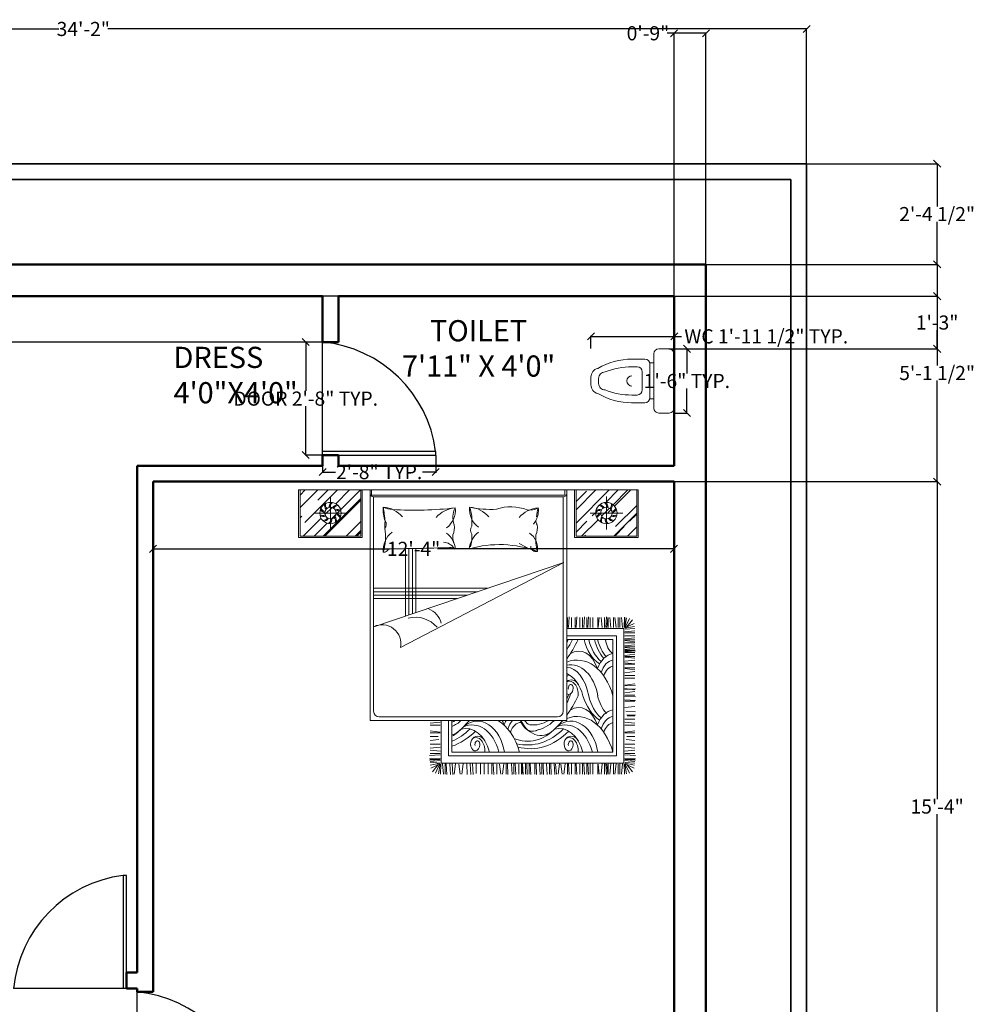
# Model space of a CAD drawing. Units: inches. Extents: x -317284 to 524, y -2236 to 1075.
# Tile 6 of 6: x 252 to 522, y 796 to 1075. Entities that reach past the tile are written whole.
import ezdxf

# ---------------------------------------------------------------- set-up
doc = ezdxf.new("R2010")
doc.units = ezdxf.units.IN
doc.header["$MEASUREMENT"] = 0
for name, color, linetype, lineweight in [('A-ANNO-DIMS', 2, 'Continuous', 18), ('A-AREA-IDEN', 7, 'Continuous', 18), ('A-DOOR', 4, 'Continuous', 25), ('A-FLOR-FIXT', 9, 'Continuous', 18), ('A-FURN', 8, 'Continuous', 18), ('A-WALL', 7, 'Continuous', 50), ('C-PROP', 3, 'Continuous', 35)]:
    doc.layers.add(name, color=color, linetype=linetype, lineweight=lineweight)
doc.styles.get("Standard").update_dxf_attribs({"font": 'arial.ttf'})
doc.dimstyles.get("Standard").update_dxf_attribs({"dimtxt": 4, "dimasz": 2, "dimexe": 0.18, "dimexo": 0.0625, "dimgap": 0.09, "dimtad": 0, "dimtih": 1, "dimtoh": 1, "dimdec": 0, "dimzin": 0, "dimdsep": 46, "dimlunit": 4, "dimtxsty": 'Standard', "dimblk": 'OBLIQUE', "dimcen": 0.09, "dimadec": 0, "dimazin": 0, "dimtfac": 1, "dimtdec": 0, "dimtofl": 0, "dimtmove": 0, "dimatfit": 3, "dimldrblk": 'OBLIQUE', "dimfxl": 1, "dimtolj": 1, "dimtzin": 0, "dimarcsym": 0})

# ---------------------------------------------------------------- blocks, each defined once
blk = doc.blocks.new('_Oblique')
at = {"color": 0, "linetype": 'ByBlock', "lineweight": -2}
blk.add_line((-0.5, -0.5), (0.5, 0.5), dxfattribs=at)
blk = doc.blocks.new('*D2')
at = {"layer": 'A-ANNO-DIMS', "color": 0, "lineweight": -2, "transparency": 16777216}
for p, q in [((290.23, 944.32), (290.23, 925.16)), ((437.73, 944.32), (437.73, 925.16)), ((290.23, 925.34), (357.2, 925.34)), ((437.73, 925.34), (370.75, 925.34))]:
    blk.add_line(p, q, dxfattribs=at)
at = {"layer": 'Defpoints', "color": 0, "transparency": 16777216}
for p in [(290.23, 944.38), (437.73, 944.38), (290.23, 925.34)]:
    blk.add_point(p, dxfattribs=at)
at = {"layer": 'A-ANNO-DIMS', "color": 0, "lineweight": -2, "transparency": 16777216, "xscale": 2, "yscale": 2, "zscale": 2, "rotation": 180}
blk.add_blockref('_Oblique', (290.23, 925.34), dxfattribs=at)
at = {"layer": 'A-ANNO-DIMS', "color": 0, "lineweight": -2, "transparency": 16777216, "xscale": 2, "yscale": 2, "zscale": 2}
blk.add_blockref('_Oblique', (437.73, 925.34), dxfattribs=at)
at = {"layer": 'A-ANNO-DIMS', "color": 0, "transparency": 16777216, "insert": (363.98, 925.34), "char_height": 4, "attachment_point": 5}
blk.add_mtext('\\A1;12\'-4"', dxfattribs=at)
blk = doc.blocks.new('SDFGHJK')
for p, q in [((282.73, 832.88), (281.73, 832.88)), ((281.73, 832.88), (281.73, 800.88)), ((282.73, 800.88), (282.73, 832.88)), ((282.73, 800.88), (250.73, 800.88))]:
    blk.add_line(p, q)
blk.add_arc((286.22, 797.51), 35.65, 97.2399, 174.5788)
blk = doc.blocks.new('A$C744D6A7D')
for p, q in [((0.0432, 0.6979), (0.4969, 0.7022)), ((0, 0.5725), (0, 0.6547)), ((0.5401, 0.659), (0.5401, 0.5725)), ((0.4969, 0.5293), (0.0432, 0.5293)), ((0.1188, 0.5293), (0.1188, 0.4969)), ((0.4213, 0.4969), (0.4213, 0.5293)), ((0.0864, 0.3427), (0.0864, 0.4537)), ((0.1188, 0.4969), (0.4213, 0.4969)), ((0.1296, 0.4969), (0.4105, 0.4969)), ((0.1944, 0.4321), (0.3457, 0.4321)), ((0.4537, 0.4537), (0.4537, 0.3427)), ((0.1512, 0.3889), (0.1512, 0.3457)), ((0.3889, 0.3889), (0.3889, 0.3457)), ((0.2377, 0), (0.3025, 0)), ((0.2701, 0.0648), (0.2485, 0.0648)), ((0.2701, 0.0648), (0.2917, 0.0648))]:
    blk.add_line(p, q)
for centre, radius, start, end in [((0.0432, 0.6547), 0.0432, 90, 180), ((0.4969, 0.659), 0.0432, 0, 90), ((0.0432, 0.5725), 0.0432, 180, 270), ((0.4969, 0.5725), 0.0432, 270, 0), ((0.1296, 0.4537), 0.0432, 90, 180), ((0.1944, 0.3889), 0.0432, 90, 180), ((0.3457, 0.3889), 0.0432, 0, 90), ((0.4105, 0.4537), 0.0432, 0, 90), ((0.6538, 0.3442), 0.5674, 179.85141, 210.37068), ((0.7683, 0.3457), 0.6171, 180, 201.56859), ((0.2701, 0.3457), 0.0432, 180, 0), ((-0.2282, 0.3457), 0.6171, 338.43141, 0), ((-0.1137, 0.3442), 0.5674, 329.62932, 0.14859), ((0.2485, 0.1188), 0.054, 180, 270), ((0.2917, 0.1188), 0.054, 270, 0), ((0.2377, 0.0756), 0.0756, 193.98485, 270), ((0.3025, 0.0756), 0.0756, 270, 346.01515)]:
    blk.add_arc(centre, radius, start, end)
blk = doc.blocks.new('A$C64B41DC1')
for p, q in [((0, 2.5079), (2.9903, 2.5079)), ((0, 2.0879), (0, 2.5079)), ((0.012, 2.4618), (0.0581, 2.5079)), ((0.012, 2.3515), (0.1684, 2.5079)), ((0.012, 2.0999), (0.012, 2.5079)), ((0.0543, 2.2213), (0.3409, 2.5079)), ((0.1689, 2.4179), (0.2589, 2.5079)), ((0.2157, 2.0999), (0.548, 2.4322)), ((0.2804, 2.1597), (0.2804, 2.4481)), ((0.3265, 2.386), (0.4484, 2.5079)), ((0.3699, 2.3332), (0.5445, 2.5079)), ((0.548, 2.5079), (0.548, 2.0999)), ((0.56, 2.5079), (0.56, 2.0879)), ((0.6301, 2.5079), (0.6301, 0.4779)), ((0.6401, 2.461), (0.6401, 2.5079)), ((0.6401, 2.5079), (2.344, 2.5079)), ((2.344, 2.461), (0.6401, 2.461)), ((0.6601, 2.4461), (1.4951, 2.4461)), ((0.6601, 2.4461), (0.6601, 0.5579)), ((1.4951, 2.4461), (0.6697, 2.4461)), ((2.3301, 2.4461), (1.4951, 2.4461)), ((2.3301, 0.5579), (2.3301, 2.4461)), ((2.344, 2.5079), (2.3601, 2.5079)), ((2.344, 2.5079), (2.344, 2.461)), ((2.3601, 2.5079), (2.3601, 2.4761)), ((2.3601, 0.4779), (2.3601, 2.5079)), ((2.4303, 2.5079), (2.4303, 2.0879)), ((2.4423, 2.5079), (2.4423, 2.0999)), ((2.4423, 2.3333), (2.6169, 2.5079)), ((2.4423, 2.2145), (2.7357, 2.5079)), ((2.4423, 2.404), (2.5354, 2.4971)), ((2.705, 2.398), (2.8149, 2.5079)), ((2.7099, 2.1597), (2.7099, 2.4481)), ((2.7691, 2.3772), (2.8998, 2.5079)), ((2.7819, 2.3646), (2.9252, 2.5079)), ((2.9783, 2.0999), (2.9783, 2.5079)), ((2.9903, 2.0879), (2.9903, 2.5079)), ((0.2299, 2.0999), (0.548, 2.418)), ((0.2311, 2.2906), (0.2937, 2.3532)), ((2.6674, 2.2756), (2.7382, 2.3464)), ((2.7914, 2.1846), (2.9783, 2.3715)), ((0.012, 2.261), (0.0275, 2.2765)), ((0.0404, 2.0999), (0.1982, 2.2578)), ((0.1362, 2.3039), (0.4246, 2.3039)), ((0.2905, 2.2539), (0.3304, 2.2938)), ((0.3405, 2.3039), (0.3605, 2.3238)), ((2.8541, 2.3039), (2.5657, 2.3039)), ((2.5849, 2.2779), (2.6158, 2.3088)), ((2.6158, 2.3088), (2.6313, 2.3243)), ((2.7249, 2.3076), (2.7512, 2.3339)), ((2.7746, 2.0999), (2.9783, 2.3036)), ((2.9144, 2.2312), (2.9783, 2.2951)), ((0.1365, 2.0999), (0.251, 2.2144)), ((0.4194, 2.0999), (0.548, 2.2285)), ((2.4423, 2.1353), (2.5382, 2.2312)), ((2.4918, 2.0999), (2.6366, 2.2447)), ((2.7831, 2.0999), (2.8678, 2.1846)), ((2.8962, 2.0999), (2.9783, 2.182)), ((0.56, 2.0879), (0, 2.0879)), ((0.548, 2.0999), (0.012, 2.0999)), ((0.4986, 2.0999), (0.548, 2.1493)), ((0.5127, 2.0999), (0.548, 2.1352)), ((2.4303, 2.0879), (2.9903, 2.0879)), ((2.4423, 2.0999), (2.9783, 2.0999)), ((2.5172, 2.0999), (2.5269, 2.1096)), ((0.9415, 1.9902), (0.9415, 1.3975)), ((0.9715, 1.9906), (0.9715, 1.4076)), ((1.0015, 1.991), (1.0015, 1.4177)), ((1.0315, 1.9916), (1.0315, 1.4279)), ((2.3349, 1.8678), (0.6613, 1.3029)), ((0.8956, 1.1191), (2.3349, 1.8678)), ((1.6636, 1.6412), (0.6601, 1.6412)), ((1.5748, 1.6112), (0.6601, 1.6112)), ((2.377, 1.295), (2.3822, 1.3891)), ((2.4451, 1.295), (2.4503, 1.3891)), ((2.5105, 1.295), (2.5157, 1.3891)), ((2.5471, 1.295), (2.5524, 1.3891)), ((2.7043, 1.295), (2.7095, 1.3891)), ((2.3665, 1.295), (2.3665, 1.3839)), ((2.4032, 1.295), (2.4032, 1.3839)), ((2.4346, 1.295), (2.4346, 1.3839)), ((2.4774, 1.2957), (2.4774, 1.3837)), ((2.5, 1.295), (2.5, 1.3839)), ((2.5367, 1.295), (2.5367, 1.3839)), ((2.5681, 1.295), (2.5681, 1.3839)), ((2.5918, 1.295), (2.5918, 1.3839)), ((2.6346, 1.2957), (2.6346, 1.3837)), ((2.6362, 1.2957), (2.6467, 1.3839)), ((2.6729, 1.295), (2.6624, 1.3839)), ((2.6938, 1.295), (2.6938, 1.3839)), ((2.7127, 1.2957), (2.7232, 1.3839)), ((2.7253, 1.295), (2.7253, 1.3839)), ((2.7494, 1.295), (2.7389, 1.3839)), ((2.7718, 1.295), (2.7718, 1.3839)), ((2.7959, 1.295), (2.7854, 1.3839)), ((2.8146, 1.2957), (2.8146, 1.3837)), ((2.8146, 1.2957), (2.8146, 1.3837)), ((2.8282, 1.295), (2.8282, 1.3839)), ((2.8282, 1.295), (2.8282, 1.3839)), ((2.8523, 1.295), (2.8418, 1.3839)), ((2.8523, 1.295), (2.8418, 1.3839)), ((2.8653, 1.2966), (2.8688, 1.3861)), ((2.8711, 1.2957), (2.8711, 1.3837)), ((2.8711, 1.2957), (2.8875, 1.3822)), ((2.8713, 1.2927), (2.954, 1.3315)), ((2.8717, 1.2884), (2.9588, 1.3058)), ((2.8765, 1.2958), (2.9132, 1.3758)), ((2.8893, 1.3011), (2.9394, 1.3636)), ((2.3601, 1.2873), (2.8639, 1.2873)), ((2.3601, 1.2233), (2.7999, 1.2233)), ((2.7999, 1.2233), (2.7999, 0.1658)), ((2.8639, 1.2873), (2.8639, 0.1018)), ((2.8716, 1.2565), (2.9605, 1.2669)), ((2.8716, 1.2212), (2.9605, 1.2212)), ((2.8723, 1.2489), (2.9603, 1.2489)), ((2.8744, 1.2817), (2.9603, 1.2869)), ((2.3601, 1.1913), (2.7679, 1.1912)), ((2.7679, 1.1912), (2.7679, 0.1978)), ((2.8716, 1.1947), (2.9605, 1.2052)), ((2.8716, 1.181), (2.9605, 1.1705)), ((2.8716, 1.1595), (2.9605, 1.1595)), ((2.8716, 1.133), (2.9605, 1.1435)), ((2.8723, 1.1872), (2.9603, 1.1872)), ((2.8716, 1.1193), (2.9605, 1.1088)), ((2.8716, 1.1035), (2.9605, 1.093)), ((2.8716, 1.0965), (2.9605, 1.0965)), ((2.8716, 1.086), (2.9657, 1.0913)), ((2.8716, 1.0756), (2.9605, 1.0756)), ((2.8716, 1.0491), (2.9605, 1.0596)), ((2.8723, 1.1255), (2.9603, 1.1255)), ((2.8723, 1.0858), (2.9605, 1.0753)), ((2.8723, 1.0416), (2.9603, 1.0416)), ((2.8716, 1.0354), (2.9605, 1.0249)), ((2.8723, 0.9987), (2.9605, 1.0092)), ((2.8723, 0.985), (2.9605, 0.9745)), ((2.8723, 0.9735), (2.9603, 0.9735)), ((2.8716, 0.9346), (2.9605, 0.9241)), ((2.8723, 0.9408), (2.9603, 0.9408)), ((2.8723, 0.8979), (2.9605, 0.9084)), ((2.8723, 0.8726), (2.9603, 0.8726)), ((2.8716, 0.7885), (2.9605, 0.799)), ((2.8716, 0.7818), (2.9657, 0.787)), ((2.8723, 0.8505), (2.9603, 0.8505)), ((2.8716, 0.7503), (2.9657, 0.7556)), ((2.8716, 0.7204), (2.9605, 0.7309)), ((2.8716, 0.6995), (2.9605, 0.6995)), ((2.8723, 0.7571), (2.9605, 0.7466)), ((2.8716, 0.689), (2.9657, 0.6838)), ((2.8716, 0.6576), (2.9657, 0.6523)), ((2.8716, 0.6471), (2.9605, 0.6471)), ((2.8716, 0.5903), (2.9605, 0.6007)), ((2.882, 0.5582), (2.9657, 0.5536)), ((2.8909, 0.5263), (2.9657, 0.5222)), ((0.6301, 0.4779), (2.3601, 0.4779)), ((0.7101, 0.5079), (2.2801, 0.5079)), ((1.2465, 0.4625), (1.1576, 0.452)), ((1.2465, 0.4365), (1.1577, 0.4365)), ((1.2542, 0.1018), (1.2542, 0.4779)), ((1.3182, 0.1658), (1.3182, 0.4779)), ((1.3502, 0.1978), (1.3502, 0.4779)), ((2.8716, 0.4877), (2.9603, 0.4877)), ((2.8716, 0.4625), (2.9605, 0.452)), ((2.8716, 0.4365), (2.9603, 0.4365)), ((2.8928, 0.5169), (2.9605, 0.5169)), ((1.2465, 0.3746), (1.1576, 0.3851)), ((1.2465, 0.3684), (1.1577, 0.3684)), ((2.8716, 0.3746), (2.9605, 0.3851)), ((2.8716, 0.3684), (2.9603, 0.3684)), ((1.2355, 0.3092), (1.1576, 0.3)), ((1.2285, 0.3357), (1.1577, 0.3357)), ((1.2457, 0.2676), (1.1577, 0.2676)), ((2.8723, 0.2676), (2.9603, 0.2676)), ((2.8826, 0.3092), (2.9605, 0.3)), ((2.8896, 0.3357), (2.9603, 0.3357)), ((1.2465, 0.1742), (1.1524, 0.169)), ((1.2457, 0.2423), (1.1576, 0.2319)), ((1.2465, 0.2057), (1.1576, 0.2161)), ((1.2465, 0.1847), (1.1576, 0.1847)), ((2.7679, 0.1978), (1.3502, 0.1978)), ((2.8716, 0.2057), (2.9605, 0.2161)), ((2.8716, 0.1847), (2.9605, 0.1847)), ((2.8716, 0.1742), (2.9657, 0.169)), ((2.8723, 0.2423), (2.9605, 0.2319)), ((1.2465, 0.1428), (1.1524, 0.1376)), ((1.2465, 0.1334), (1.1524, 0.1281)), ((1.2465, 0.1323), (1.1576, 0.1323)), ((1.2465, 0.1323), (1.1576, 0.1323)), ((1.2465, 0.1), (1.1576, 0.1105)), ((1.2465, 0.1229), (1.1588, 0.1168)), ((1.2464, 0.1007), (1.1592, 0.0833)), ((1.2468, 0.0964), (1.1641, 0.0576)), ((1.2288, 0.088), (1.1787, 0.0255)), ((1.2415, 0.0933), (1.2049, 0.0133)), ((1.247, 0.0934), (1.2306, 0.0069)), ((1.2527, 0.0925), (1.2493, 0.003)), ((2.8639, 0.1018), (1.2542, 0.1018)), ((1.2658, 0.0941), (1.2762, 0.0052)), ((1.2899, 0.0941), (1.2899, 0.0052)), ((1.2999, 0.0941), (1.3051, 0)), ((2.7999, 0.1658), (1.3182, 0.1658)), ((1.3313, 0.0941), (1.3365, 0)), ((1.3523, 0.0941), (1.3575, 0)), ((1.3804, 0.0941), (1.3699, 0.0052)), ((1.4119, 0.0934), (1.4223, 0.0052)), ((1.4485, 0.0941), (1.438, 0.0052)), ((1.48, 0.0941), (1.4852, 0)), ((1.5114, 0.0941), (1.5166, 0)), ((1.5323, 0.0941), (1.5376, 0)), ((1.5638, 0.0941), (1.5638, 0.0105)), ((1.6021, 0.0941), (1.6021, 0.0052)), ((1.6336, 0.0941), (1.6336, 0.0052)), ((1.6702, 0.0941), (1.6702, 0.0052)), ((1.7017, 0.0941), (1.7017, 0.0052)), ((1.7122, 0.0941), (1.7174, 0)), ((1.7445, 0.0934), (1.7445, 0.0054)), ((1.7698, 0.0934), (1.7803, 0.0052)), ((1.8065, 0.0941), (1.796, 0.0052)), ((1.8274, 0.0941), (1.8274, 0.0052)), ((1.8379, 0.0941), (1.8431, 0)), ((1.8746, 0.0941), (1.8798, 0)), ((1.8955, 0.0941), (1.8955, 0.0052)), ((1.906, 0.0941), (1.9113, 0)), ((1.9384, 0.0934), (1.9384, 0.0054)), ((1.9609, 0.0941), (1.9609, 0.0052)), ((1.9636, 0.0934), (1.9741, 0.0052)), ((1.9714, 0.0941), (1.9766, 0)), ((1.9976, 0.0941), (1.9976, 0.0052)), ((2.0081, 0.0941), (2.0133, 0)), ((2.029, 0.0941), (2.029, 0.0052)), ((2.0395, 0.0941), (2.0447, 0)), ((2.0797, 0.0941), (2.0797, 0.0052)), ((2.0902, 0.0941), (2.0954, 0)), ((2.1216, 0.0941), (2.1269, 0)), ((2.1412, 0.0941), (2.1412, 0.0052)), ((2.1517, 0.0941), (2.1569, 0)), ((2.1831, 0.0941), (2.1884, 0)), ((2.2093, 0.0941), (2.2093, 0.0052)), ((2.2198, 0.0941), (2.225, 0)), ((2.2512, 0.0941), (2.2565, 0)), ((2.2603, 0.0934), (2.2707, 0.0052)), ((2.2969, 0.0941), (2.2864, 0.0052)), ((2.3089, 0.0934), (2.3193, 0.0052)), ((2.3455, 0.0941), (2.3351, 0.0052)), ((2.3665, 0.0941), (2.3665, 0.0052)), ((2.377, 0.0941), (2.3822, 0)), ((2.4032, 0.0941), (2.4032, 0.0052)), ((2.4346, 0.0941), (2.4346, 0.0052)), ((2.4451, 0.0941), (2.4503, 0)), ((2.4774, 0.0934), (2.4774, 0.0054)), ((2.5, 0.0941), (2.5, 0.0052)), ((2.5105, 0.0941), (2.5157, 0)), ((2.5367, 0.0941), (2.5367, 0.0052)), ((2.5471, 0.0941), (2.5524, 0)), ((2.5681, 0.0941), (2.5681, 0.0052)), ((2.5918, 0.0941), (2.5918, 0.0052)), ((2.6346, 0.0934), (2.6346, 0.0054)), ((2.6362, 0.0934), (2.6467, 0.0052)), ((2.6729, 0.0941), (2.6624, 0.0052)), ((2.6938, 0.0941), (2.6938, 0.0052)), ((2.7043, 0.0941), (2.7095, 0)), ((2.7127, 0.0934), (2.7232, 0.0052)), ((2.7253, 0.0941), (2.7253, 0.0052)), ((2.7494, 0.0941), (2.7389, 0.0052)), ((2.7718, 0.0941), (2.7718, 0.0052)), ((2.7959, 0.0941), (2.7854, 0.0052)), ((2.8146, 0.0934), (2.8146, 0.0054)), ((2.8282, 0.0941), (2.8282, 0.0052)), ((2.8523, 0.0941), (2.8418, 0.0052)), ((2.8653, 0.0925), (2.8688, 0.003)), ((2.8711, 0.0934), (2.8875, 0.0069)), ((2.8713, 0.0964), (2.954, 0.0576)), ((2.8716, 0.1428), (2.9657, 0.1376)), ((2.8716, 0.1334), (2.9657, 0.1281)), ((2.8716, 0.1323), (2.9605, 0.1323)), ((2.8716, 0.1229), (2.9593, 0.1168)), ((2.8717, 0.1007), (2.9588, 0.0833)), ((2.8744, 0.1074), (2.9603, 0.1022)), ((2.8765, 0.0933), (2.9132, 0.0133)), ((2.8893, 0.088), (2.9394, 0.0255))]:
    blk.add_line(p, q)
at = {"ltscale": 10}
for p, q in [((1.4859, 1.5812), (0.6601, 1.5812)), ((1.397, 1.5512), (0.6601, 1.5512))]:
    blk.add_line(p, q, dxfattribs=at)
for centre, radius in [((0.2804, 2.3039), 0.0942), ((0.2804, 2.3039), 0.051), ((2.7099, 2.3039), 0.0942), ((2.7099, 2.3039), 0.051)]:
    blk.add_circle(centre, radius)
for centre, radius, start, end in [((0.6601, 2.4761), 0.03, 180, 270), ((2.3301, 2.4761), 0.03, 270, 0), ((0.2417, 2.3614), 0.0462, 196.30017, 256.53802), ((0.2887, 2.3745), 0.0605, 172.17003, 218.48975), ((0.2828, 2.3731), 0.0462, 160.30017, 220.53802), ((0.3286, 2.3561), 0.0605, 136.17003, 182.48975), ((0.3231, 2.3585), 0.0462, 124.30017, 184.53802), ((0.3501, 2.3178), 0.0605, 100.17003, 146.48975), ((0.347, 2.323), 0.0462, 88.30017, 148.53802), ((1.0526, 2.3302), 0.3085, 175.30484, 198.69419), ((-0.8702, 2.0941), 1.6364, 4.80985, 9.18918), ((0.8579, 2.6278), 0.2948, 247.51785, 264.26696), ((0.728, 2.111), 0.245, 40.4189, 85.9871), ((1.0164, 5.7096), 3.3803, 266.81337, 276.16021), ((1.3963, 2.1044), 0.245, 94.0129, 139.5811), ((1.1858, 2.3288), 0.1943, 306.5711, 5.88998), ((1.5348, 2.2652), 0.1767, 151.77364, 201.69827), ((1.6986, 2.3355), 0.1943, 174.11002, 233.4289), ((1.1481, 2.2311), 0.3783, 353.49469, 19.18669), ((1.6871, 3.192), 0.8561, 257.74383, 273.62843), ((1.4882, 2.111), 0.245, 40.4189, 85.9871), ((1.8674, 1.9709), 0.3878, 68.20259, 108.9817), ((2.1269, 2.1044), 0.245, 94.0129, 139.5811), ((2.0342, 2.4856), 0.1563, 261.59582, 298.90918), ((1.9165, 2.3288), 0.1943, 333.73715, 5.88998), ((2.6058, 2.2028), 0.517, 163.60457, 172.3273), ((2.6433, 2.323), 0.0462, 31.46198, 91.69983), ((2.6402, 2.3178), 0.0605, 33.51025, 79.82997), ((2.6672, 2.3585), 0.0462, 355.46198, 55.69983), ((2.6617, 2.3561), 0.0605, 357.51025, 43.82997), ((2.7075, 2.3731), 0.0462, 319.46198, 19.69983), ((2.7016, 2.3745), 0.0605, 321.51025, 7.82997), ((2.7486, 2.3614), 0.0462, 283.46198, 343.69983), ((0.2153, 2.3276), 0.0462, 232.30017, 292.53802), ((0.2158, 2.3336), 0.0605, 244.17003, 290.48975), ((0.2457, 2.3659), 0.0605, 208.17003, 254.48975), ((0.2138, 2.2848), 0.0462, 268.30017, 328.53802), ((0.2107, 2.29), 0.0605, 280.17003, 326.48975), ((0.2779, 2.2347), 0.0462, 340.30017, 40.53802), ((0.272, 2.2333), 0.0605, 352.17003, 38.48975), ((0.3449, 2.2742), 0.0605, 64.17003, 110.48975), ((0.3455, 2.2802), 0.0462, 52.30017, 112.53802), ((0.3191, 2.2464), 0.0462, 16.30017, 76.53802), ((0.3151, 2.2419), 0.0605, 28.17003, 74.48975), ((2.6448, 2.2802), 0.0462, 67.46198, 127.69983), ((2.6454, 2.2742), 0.0605, 69.51025, 115.82997), ((2.6752, 2.2419), 0.0605, 105.51025, 151.82997), ((2.6712, 2.2464), 0.0462, 103.46198, 163.69983), ((2.7182, 2.2333), 0.0605, 141.51025, 187.82997), ((2.7123, 2.2347), 0.0462, 139.46198, 199.69983), ((2.7796, 2.29), 0.0605, 213.51025, 259.82997), ((2.7765, 2.2848), 0.0462, 211.46198, 271.69983), ((2.7744, 2.3336), 0.0605, 249.51025, 295.82997), ((2.775, 2.3276), 0.0462, 247.46198, 307.69983), ((2.7446, 2.3659), 0.0605, 285.51025, 331.82997), ((0.2377, 2.2493), 0.0462, 304.30017, 4.53802), ((0.2322, 2.2517), 0.0605, 316.17003, 2.48975), ((0.2688, 2.0945), 0.4956, 344.0243, 8.70709), ((0.7274, 2.2013), 0.0446, 314.4736, 42.17134), ((-1.6008, 2.277), 2.3618, 357.39054, 358.88764), ((1.204, 2.1778), 0.1681, 337.01697, 7.53676), ((1.5671, 2.1546), 0.0547, 142.08329, 220.902), ((1.9165, 2.3288), 0.1943, 320.94042, 333.73715), ((2.1347, 2.2313), 0.0459, 165.35061, 223.26844), ((1.9346, 2.1778), 0.1681, 337.01697, 7.53676), ((2.7581, 2.2517), 0.0605, 177.51025, 223.82997), ((2.7526, 2.2493), 0.0462, 175.46198, 235.69983), ((0.9385, 1.978), 0.1943, 126.5711, 185.88998), ((1.1858, 1.9714), 0.1943, 4.31813, 53.4289), ((1.5415, 2.0969), 0.1834, 175.22328, 196.23004), ((1.7059, 1.9714), 0.204, 127.11975, 175.09005), ((1.1965, 2.0983), 0.3299, 343.79543, 3.55541), ((1.9394, 1.991), 0.1651, 351.26213, 55.75721), ((2.4617, 2.0719), 0.3745, 173.82958, 196.4356), ((0.7246, 18.8439), 16.8552, 270.17399, 272.05214), ((1.2687, 1.9248), 0.1223, 33.62799, 86.47438), ((1.3401, 1.9404), 0.0603, 49.09906, 101.37023), ((1.7676, 1.0629), 0.9631, 69.65065, 105.96307), ((2.2748, 2.5795), 0.6373, 238.34989, 254.31375), ((2.0911, 2.0123), 0.0478, 179.77267, 283.80184), ((0.7417, 2.0149), 0.057, 273.47085, 328.54118), ((0.728, 2.2025), 0.245, 274.0129, 278.34166), ((1.0747, 1.2871), 0.1871, 14.1863, 69.12121), ((0.7347, 1.1553), 0.1649, 347.31088, 116.44537), ((1.0274, 1.1334), 0.2527, 40.62904, 104.37123), ((0.7101, 0.5579), 0.05, 180, 270), ((2.2801, 0.5579), 0.05, 270, 0)]:
    blk.add_arc(centre, radius, start, end)
for centre, major_axis, ratio, start_param, end_param in [((1.9938, 1.6262), (0, -0.7531), 0.68, 0.797284, 0.954936), ((2.0643, 1.466), (0, -0.5322), 0.68, 7.239912, 7.311536), ((1.9052, 1.7397), (0, -0.9842), 0.68, 0.74745, 0.979724), ((2.7455, 1.3081), (0, 0.3614), 0.68, 1.900046, 2.742661), ((2.7868, 1.3081), (0, 0.3614), 0.68, 1.900046, 2.614747), ((2.8372, 1.3081), (0, 0.3614), 0.68, 1.900046, 2.479658), ((2.8607, 1.3211), (0, 0.3614), 0.68, 1.938265, 2.479658), ((2.8057, 1.2079), (0, -0.1524), 0.68, 4.821745, 5.895886), ((2.4513, 0.5069), (0, 0.502), 0.68, 5.095327, 6.553458), ((2.4665, 0.8216), (0, -0.2664), 0.68, 2.006169, 3.565187), ((2.7862, 0.8069), (0, -0.2615), 0.68, 3.244645, 4.205018), ((2.396, 0.6032), (0, 0.3641), 0.68, -1.3172, 0.145284), ((2.7784, 0.8289), (0, -0.1802), 0.68, 3.227058, 4.318474), ((2.7821, 0.7971), (0, -0.1589), 0.68, 3.272942, 4.229533), ((2.3507, 0.5642), (0.0073, 0.3819), 0.56205, -1.21172, -0.009991), ((2.2964, 0.5771), (0, -0.3263), 0.68, 1.938944, 2.850232), ((2.0403, 1.6015), (0, -0.8763), 0.68, 6.849801, 6.887077), ((2.4005, 0.7132), (0, -0.1214), 0.68, 2.284368, 3.652258), ((2.3834, 0.7081), (0, 0.1147), 0.68, 4.593909, 6.585576), ((2.3961, 0.7628), (0, -0.0317), 0.68, 1.462497, 5.046281), ((2.3774, 0.7653), (0, -0.0593), 0.68, 5.841311, 7.755362), ((1.9938, 1.1295), (-0.0678, 0.7439), 0.610498, 3.917146, 4.063997), ((2.0643, 0.9693), (0, -0.5322), 0.68, 7.239912, 7.336618), ((1.9052, 1.243), (0, -0.9842), 0.68, 0.74745, 0.979724), ((2.7455, 0.8114), (-0.0599, 0.3735), 0.695517, 1.775813, 2.548612), ((2.7868, 0.8114), (0, 0.3614), 0.68, 1.900046, 2.614747), ((2.8607, 0.8243), (0, 0.3614), 0.68, 1.938265, 2.479658), ((2.4665, 0.3249), (0, -0.2664), 0.68, 2.006169, 3.565187), ((2.4513, 0.0102), (0, 0.502), 0.68, 5.095327, 6.553458), ((2.7862, 0.3102), (0, -0.2615), 0.68, 3.244645, 4.205018), ((1.242, 0.9693), (0, -0.5322), 0.68, 6.586764, 6.677612), ((1.1714, 1.1295), (-0.1157, 0.7241), 0.59432, 3.291697, 3.50733), ((1.0828, 1.243), (0, -0.9842), 0.68, 0.565948, 0.680366), ((1.5283, 0.0674), (0, -0.3703), 0.68, 1.930561, 3.464283), ((1.5736, 0.1065), (0, 0.3641), 0.68, -1.3172, 0.476403), ((1.6289, 0.0102), (0, 0.502), 0.68, 6.655152, 6.661293), ((1.6289, 0.0102), (0, 0.502), 0.68, 5.095327, 5.911219), ((1.6442, 0.3249), (0, -0.2664), 0.68, 2.006169, 2.182797), ((1.9638, 0.3102), (0, -0.2615), 0.68, 4.015924, 4.205018), ((1.956, 0.3322), (0, -0.1802), 0.68, 3.770744, 4.318474), ((1.9597, 0.3004), (0, -0.1589), 0.68, 3.14258, 4.229533), ((2.0606, 0.5616), (0, -0.1803), 0.68, 5.194792, 5.929328), ((2.0606, 0.5616), (0, -0.1803), 0.68, 5.194792, 6.723255), ((2.1315, 0.6603), (0, -0.3155), 0.68, 5.328638, 6.949396), ((2.0549, 0.5656), (0, -0.1303), 0.68, 5.450951, 6.054641), ((2.0643, 0.9693), (0, -0.5322), 0.68, 6.20013, 6.677612), ((1.9938, 1.1295), (-0.0678, 0.7439), 0.610498, 3.199135, 3.592282), ((1.9052, 1.243), (0, -0.9842), 0.68, 0.565948, 0.680366), ((2.3507, 0.0674), (0, -0.3703), 0.68, 1.930561, 3.464283), ((2.396, 0.1065), (0, 0.3641), 0.68, -1.3172, 0.476403), ((2.4513, 0.0102), (0, 0.502), 0.68, 6.655152, 6.661293), ((2.7784, 0.3322), (0, -0.1802), 0.68, 3.227058, 4.318474), ((2.7821, 0.3004), (0, -0.1589), 0.68, 3.272942, 4.229533), ((1.1933, 0.9181), (0, -0.624), 0.68, 0.378672, 0.625379), ((1.3091, 0.6603), (0, -0.3155), 0.68, 6.475719, 6.949396), ((1.1911, 1.1066), (0, 0.8458), 0.68, 3.421828, 3.728616), ((1.2179, 1.1047), (0, -0.8763), 0.68, 6.507006, 6.887077), ((1.474, 0.0804), (0, -0.3263), 0.68, 1.938944, 3.339184), ((1.5781, 0.2165), (0, -0.1214), 0.68, 2.284368, 3.726131), ((2.0157, 0.9181), (0, -0.624), 0.68, -0.280078, 0.625379), ((2.0135, 1.1066), (0, 0.8458), 0.68, 2.978727, 3.728616), ((2.0403, 1.1047), (0, -0.8763), 0.68, 6.099302, 6.887077), ((2.2964, 0.0804), (0, -0.3263), 0.68, 1.938944, 3.339184), ((2.4005, 0.2165), (0, -0.1214), 0.68, 2.284368, 3.726131), ((1.555, 0.2685), (0, -0.0593), 0.68, 3.732151, 7.755362), ((1.561, 0.2114), (0, 0.1147), 0.68, 4.593909, 6.647252), ((1.5737, 0.2661), (0, -0.0317), 0.68, 1.462497, 5.046281), ((2.3774, 0.2685), (0, -0.0593), 0.68, 3.732151, 7.755362), ((2.3834, 0.2114), (0, 0.1147), 0.68, 4.593909, 6.647252), ((2.3961, 0.2661), (0, -0.0317), 0.68, 1.462497, 5.046281)]:
    blk.add_ellipse(centre, major_axis=major_axis, ratio=ratio, start_param=start_param, end_param=end_param)
blk = doc.blocks.new('*D14')
at = {"layer": 'A-ANNO-DIMS', "color": 0, "lineweight": -2, "transparency": 16777216}
for p, q in [((65.73, 1034.44), (65.73, 1072.72)), ((65.73, 1072.54), (263.52, 1072.54)), ((475.23, 1072.54), (277.44, 1072.54)), ((475.23, 1034.44), (475.23, 1072.72))]:
    blk.add_line(p, q, dxfattribs=at)
at = {"layer": 'Defpoints', "color": 0, "transparency": 16777216}
for p in [(475.23, 1072.54), (65.73, 1034.38), (475.23, 1034.38)]:
    blk.add_point(p, dxfattribs=at)
at = {"layer": 'A-ANNO-DIMS', "color": 0, "lineweight": -2, "transparency": 16777216, "xscale": 2, "yscale": 2, "zscale": 2, "rotation": 180}
blk.add_blockref('_Oblique', (65.73, 1072.54), dxfattribs=at)
at = {"layer": 'A-ANNO-DIMS', "color": 0, "lineweight": -2, "transparency": 16777216, "xscale": 2, "yscale": 2, "zscale": 2}
blk.add_blockref('_Oblique', (475.23, 1072.54), dxfattribs=at)
at = {"layer": 'A-ANNO-DIMS', "color": 0, "transparency": 16777216, "insert": (270.48, 1072.54), "char_height": 4, "attachment_point": 5}
blk.add_mtext('\\A1;34\'-2"', dxfattribs=at)
blk = doc.blocks.new('*D17')
at = {"layer": 'A-ANNO-DIMS', "color": 0, "lineweight": -2, "transparency": 16777216}
for p, q in [((338.16, 983.88), (333.25, 983.88)), ((333.43, 983.88), (333.43, 970.04)), ((333.43, 951.88), (333.43, 965.72)), ((338.16, 951.88), (333.25, 951.88))]:
    blk.add_line(p, q, dxfattribs=at)
at = {"layer": 'Defpoints', "color": 0, "transparency": 16777216}
for p in [(338.23, 983.88), (333.43, 951.88), (338.23, 951.88)]:
    blk.add_point(p, dxfattribs=at)
at = {"layer": 'A-ANNO-DIMS', "color": 0, "lineweight": -2, "transparency": 16777216, "xscale": 2, "yscale": 2, "zscale": 2}
for p, rotation in [((333.43, 983.88), 90), ((333.43, 951.88), 270)]:
    blk.add_blockref('_Oblique', p, dxfattribs=dict(at, rotation=rotation))
at = {"layer": 'A-ANNO-DIMS', "color": 0, "transparency": 16777216, "insert": (333.43, 967.88), "char_height": 4, "attachment_point": 5}
blk.add_mtext('\\A1;DOOR 2\'-8" TYP.', dxfattribs=at)
blk = doc.blocks.new('*D18')
at = {"layer": 'A-ANNO-DIMS', "color": 0, "lineweight": -2, "transparency": 16777216}
for p, q in [((338.23, 951.82), (338.23, 946.9)), ((370.23, 951.82), (370.23, 946.9)), ((338.23, 947.08), (341.91, 947.08)), ((370.23, 947.08), (366.54, 947.08))]:
    blk.add_line(p, q, dxfattribs=at)
at = {"layer": 'Defpoints', "color": 0, "transparency": 16777216}
for p in [(338.23, 951.88), (370.23, 951.88), (370.23, 947.08)]:
    blk.add_point(p, dxfattribs=at)
at = {"layer": 'A-ANNO-DIMS', "color": 0, "lineweight": -2, "transparency": 16777216, "xscale": 2, "yscale": 2, "zscale": 2, "rotation": 180}
blk.add_blockref('_Oblique', (338.23, 947.08), dxfattribs=at)
at = {"layer": 'A-ANNO-DIMS', "color": 0, "lineweight": -2, "transparency": 16777216, "xscale": 2, "yscale": 2, "zscale": 2}
blk.add_blockref('_Oblique', (370.23, 947.08), dxfattribs=at)
at = {"layer": 'A-ANNO-DIMS', "color": 0, "transparency": 16777216, "insert": (354.23, 947.08), "char_height": 4, "attachment_point": 5}
blk.add_mtext('\\A1;2\'-8" TYP.', dxfattribs=at)
blk = doc.blocks.new('*D21')
at = {"layer": 'A-ANNO-DIMS', "color": 0, "lineweight": -2, "transparency": 16777216}
for p, q in [((414.17, 982.03), (414.17, 985.69)), ((414.17, 985.51), (437.8, 985.51)), ((437.8, 982.03), (437.8, 985.69)), ((437.8, 985.51), (439.8, 985.51))]:
    blk.add_line(p, q, dxfattribs=at)
at = {"layer": 'Defpoints', "color": 0, "transparency": 16777216}
for p in [(437.8, 985.51), (414.17, 981.97), (437.8, 981.97)]:
    blk.add_point(p, dxfattribs=at)
at = {"layer": 'A-ANNO-DIMS', "color": 0, "lineweight": -2, "transparency": 16777216, "xscale": 2, "yscale": 2, "zscale": 2, "rotation": 180}
blk.add_blockref('_Oblique', (414.17, 985.51), dxfattribs=at)
at = {"layer": 'A-ANNO-DIMS', "color": 0, "lineweight": -2, "transparency": 16777216, "xscale": 2, "yscale": 2, "zscale": 2}
blk.add_blockref('_Oblique', (437.8, 985.51), dxfattribs=at)
at = {"layer": 'A-ANNO-DIMS', "color": 0, "transparency": 16777216, "insert": (463.81, 985.51), "char_height": 4, "attachment_point": 5}
blk.add_mtext('\\A1;WC 1\'-11 1/2" TYP.', dxfattribs=at)
blk = doc.blocks.new('*D22')
at = {"layer": 'A-ANNO-DIMS', "color": 0, "lineweight": -2, "transparency": 16777216}
for p, q in [((437.86, 981.97), (441.52, 981.97)), ((441.34, 981.97), (441.34, 975.01)), ((441.34, 963.79), (441.34, 970.75)), ((437.86, 963.79), (441.52, 963.79))]:
    blk.add_line(p, q, dxfattribs=at)
at = {"layer": 'Defpoints', "color": 0, "transparency": 16777216}
for p in [(437.8, 981.97), (437.8, 963.79), (441.34, 963.79)]:
    blk.add_point(p, dxfattribs=at)
at = {"layer": 'A-ANNO-DIMS', "color": 0, "lineweight": -2, "transparency": 16777216, "xscale": 2, "yscale": 2, "zscale": 2}
for p, rotation in [((441.34, 981.97), 90), ((441.34, 963.79), 270)]:
    blk.add_blockref('_Oblique', p, dxfattribs=dict(at, rotation=rotation))
at = {"layer": 'A-ANNO-DIMS', "color": 0, "transparency": 16777216, "insert": (441.34, 972.88), "char_height": 4, "attachment_point": 5}
blk.add_mtext('\\A1;1\'-6" TYP.', dxfattribs=at)
blk = doc.blocks.new('*D38')
at = {"layer": 'A-ANNO-DIMS', "color": 0, "lineweight": -2, "transparency": 16777216}
for p, q in [((475.29, 1034.38), (512.36, 1034.38)), ((512.18, 1034.38), (512.18, 1022.29)), ((512.18, 1005.88), (512.18, 1017.97)), ((446.79, 1005.88), (512.36, 1005.88))]:
    blk.add_line(p, q, dxfattribs=at)
at = {"layer": 'Defpoints', "color": 0, "transparency": 16777216}
for p in [(475.23, 1034.38), (512.18, 1034.38), (446.73, 1005.88)]:
    blk.add_point(p, dxfattribs=at)
at = {"layer": 'A-ANNO-DIMS', "color": 0, "lineweight": -2, "transparency": 16777216, "xscale": 2, "yscale": 2, "zscale": 2}
for p, rotation in [((512.18, 1034.38), 90), ((512.18, 1005.88), 270)]:
    blk.add_blockref('_Oblique', p, dxfattribs=dict(at, rotation=rotation))
at = {"layer": 'A-ANNO-DIMS', "color": 0, "transparency": 16777216, "insert": (512.18, 1020.13), "char_height": 4, "attachment_point": 5}
blk.add_mtext('\\A1;2\'-4 1/2"', dxfattribs=at)
blk = doc.blocks.new('*D40')
at = {"layer": 'A-ANNO-DIMS', "color": 0, "lineweight": -2, "transparency": 16777216}
for p, q in [((437.79, 944.38), (512.36, 944.38)), ((512.18, 944.38), (512.18, 854.51)), ((512.18, 760.38), (512.18, 850.25)), ((437.79, 760.38), (512.36, 760.38))]:
    blk.add_line(p, q, dxfattribs=at)
at = {"layer": 'Defpoints', "color": 0, "transparency": 16777216}
for p in [(437.73, 944.38), (512.18, 944.38), (437.73, 760.38)]:
    blk.add_point(p, dxfattribs=at)
at = {"layer": 'A-ANNO-DIMS', "color": 0, "lineweight": -2, "transparency": 16777216, "xscale": 2, "yscale": 2, "zscale": 2}
for p, rotation in [((512.18, 944.38), 90), ((512.18, 760.38), 270)]:
    blk.add_blockref('_Oblique', p, dxfattribs=dict(at, rotation=rotation))
at = {"layer": 'A-ANNO-DIMS', "color": 0, "transparency": 16777216, "insert": (512.18, 852.38), "char_height": 4, "attachment_point": 5}
blk.add_mtext('\\A1;15\'-4"', dxfattribs=at)
blk = doc.blocks.new('*D41')
at = {"layer": 'A-ANNO-DIMS', "color": 0, "lineweight": -2, "transparency": 16777216}
for p, q in [((446.79, 1005.88), (512.36, 1005.88)), ((512.18, 1005.88), (512.18, 977.29)), ((512.18, 944.38), (512.18, 972.97)), ((437.79, 944.38), (512.36, 944.38))]:
    blk.add_line(p, q, dxfattribs=at)
at = {"layer": 'Defpoints', "color": 0, "transparency": 16777216}
for p in [(446.73, 1005.88), (512.18, 1005.88), (437.73, 944.38)]:
    blk.add_point(p, dxfattribs=at)
at = {"layer": 'A-ANNO-DIMS', "color": 0, "lineweight": -2, "transparency": 16777216, "xscale": 2, "yscale": 2, "zscale": 2}
for p, rotation in [((512.18, 1005.88), 90), ((512.18, 944.38), 270)]:
    blk.add_blockref('_Oblique', p, dxfattribs=dict(at, rotation=rotation))
at = {"layer": 'A-ANNO-DIMS', "color": 0, "transparency": 16777216, "insert": (512.18, 975.13), "char_height": 4, "attachment_point": 5}
blk.add_mtext('\\A1;5\'-1 1/2"', dxfattribs=at)
blk = doc.blocks.new('*D52')
at = {"layer": 'A-ANNO-DIMS', "color": 0, "lineweight": -2, "transparency": 16777216}
for p, q in [((437.79, 996.88), (512.36, 996.88)), ((512.18, 996.88), (512.18, 991.56)), ((512.18, 981.97), (512.18, 987.29)), ((436.26, 981.97), (512.36, 981.97))]:
    blk.add_line(p, q, dxfattribs=at)
at = {"layer": 'Defpoints', "color": 0, "transparency": 16777216}
for p in [(437.73, 996.88), (436.2, 981.97), (512.18, 981.97)]:
    blk.add_point(p, dxfattribs=at)
at = {"layer": 'A-ANNO-DIMS', "color": 0, "lineweight": -2, "transparency": 16777216, "xscale": 2, "yscale": 2, "zscale": 2}
for p, rotation in [((512.18, 996.88), 90), ((512.18, 981.97), 270)]:
    blk.add_blockref('_Oblique', p, dxfattribs=dict(at, rotation=rotation))
at = {"layer": 'A-ANNO-DIMS', "color": 0, "transparency": 16777216, "insert": (512.18, 989.42), "char_height": 4, "attachment_point": 5}
blk.add_mtext('\\A1;1\'-3"', dxfattribs=at)
blk = doc.blocks.new('*D53')
at = {"layer": 'A-ANNO-DIMS', "color": 0, "lineweight": -2, "transparency": 16777216}
for p, q in [((342.66, 996.88), (28.6, 996.88)), ((28.78, 996.88), (28.78, 992.48)), ((28.78, 983.88), (28.78, 988.28)), ((342.66, 983.88), (28.6, 983.88))]:
    blk.add_line(p, q, dxfattribs=at)
at = {"layer": 'Defpoints', "color": 0, "transparency": 16777216}
for p in [(342.73, 996.88), (28.78, 983.88), (342.73, 983.88)]:
    blk.add_point(p, dxfattribs=at)
at = {"layer": 'A-ANNO-DIMS', "color": 0, "lineweight": -2, "transparency": 16777216, "xscale": 2, "yscale": 2, "zscale": 2}
for p, rotation in [((28.78, 996.88), 90), ((28.78, 983.88), 270)]:
    blk.add_blockref('_Oblique', p, dxfattribs=dict(at, rotation=rotation))
at = {"layer": 'A-ANNO-DIMS', "color": 0, "transparency": 16777216, "insert": (28.78, 990.38), "char_height": 4, "attachment_point": 5}
blk.add_mtext('\\A1;1\'-1"', dxfattribs=at)
blk = doc.blocks.new('*D54')
at = {"layer": 'A-ANNO-DIMS', "color": 0, "lineweight": -2, "transparency": 16777216}
for p, q in [((437.73, 1071.33), (435.73, 1071.33)), ((437.73, 996.94), (437.73, 1071.51)), ((446.73, 1071.33), (437.73, 1071.33)), ((446.73, 1005.94), (446.73, 1071.51))]:
    blk.add_line(p, q, dxfattribs=at)
at = {"layer": 'Defpoints', "color": 0, "transparency": 16777216}
for p in [(437.73, 1071.33), (446.73, 1005.88), (437.73, 996.88)]:
    blk.add_point(p, dxfattribs=at)
at = {"layer": 'A-ANNO-DIMS', "color": 0, "lineweight": -2, "transparency": 16777216, "xscale": 2, "yscale": 2, "zscale": 2, "rotation": 180}
blk.add_blockref('_Oblique', (437.73, 1071.33), dxfattribs=at)
at = {"layer": 'A-ANNO-DIMS', "color": 0, "lineweight": -2, "transparency": 16777216, "xscale": 2, "yscale": 2, "zscale": 2}
blk.add_blockref('_Oblique', (446.73, 1071.33), dxfattribs=at)
at = {"layer": 'A-ANNO-DIMS', "color": 0, "transparency": 16777216, "insert": (430.32, 1071.33), "char_height": 4, "attachment_point": 5}
blk.add_mtext('\\A1;0\'-9"', dxfattribs=at)

msp = doc.modelspace()

# ---------------------------------------------------------------- linework, layer by layer
at = {"layer": 'A-WALL'}
for p, q in [((103.23, 1005.88), (254.23, 1005.88)), ((254.23, 1005.88), (290.23, 1005.88)), ((290.23, 1005.88), (338.23, 1005.88)), ((338.23, 1005.88), (342.73, 1005.88)), ((342.73, 1005.88), (437.73, 1005.88)), ((437.73, 1005.88), (446.73, 1005.88)), ((446.73, 1005.88), (446.73, 996.88)), ((103.23, 996.88), (254.23, 996.88)), ((254.23, 996.88), (290.23, 996.88)), ((290.23, 996.88), (338.23, 996.88)), ((338.23, 996.88), (338.23, 983.88)), ((342.73, 996.88), (437.73, 996.88)), ((342.73, 983.88), (342.73, 996.88)), ((437.73, 996.88), (437.73, 948.88)), ((446.73, 996.88), (446.73, 948.88)), ((342.73, 983.88), (338.23, 983.88)), ((342.73, 951.88), (338.23, 951.88)), ((338.23, 951.88), (338.23, 948.88)), ((342.73, 948.88), (342.73, 951.88)), ((338.23, 948.88), (285.73, 948.88)), ((285.73, 948.88), (285.73, 805.38)), ((437.73, 948.88), (342.73, 948.88)), ((446.73, 948.88), (446.73, 944.38)), ((437.73, 944.38), (290.23, 944.38)), ((290.23, 944.38), (290.23, 800.88)), ((437.73, 944.38), (437.73, 764.88)), ((446.73, 944.38), (446.73, 805.38)), ((285.73, 805.38), (282.73, 805.38)), ((282.73, 805.38), (282.73, 800.88)), ((446.73, 805.38), (446.73, 587.03)), ((285.73, 800.88), (282.73, 800.88)), ((285.73, 800.88), (285.73, 799.88)), ((290.23, 800.88), (290.23, 799.88)), ((290.23, 799.88), (285.73, 799.88))]:
    msp.add_line(p, q, dxfattribs=at)
at = {"layer": 'C-PROP'}
for points in [[(475.23, 1034.38), (475.23, 414.53), (65.73, 414.53), (65.73, 1034.38)], [(470.73, 1029.88), (470.73, 419.03), (70.23, 419.03), (70.23, 1029.88)]]:
    msp.add_lwpolyline(points, close=True, dxfattribs=at)

# ---------------------------------------------------------------- block references
at = {"layer": 'A-DOOR', "rotation": 270}
for p in [(-462.65, 1234.61), (-515.15, 1050.61)]:
    msp.add_blockref('SDFGHJK', p, dxfattribs=at)
at = {"layer": 'A-DOOR'}
msp.add_blockref('SDFGHJK', (0, 0), dxfattribs=at)
at = {"layer": 'A-FLOR-FIXT', "xscale": 33.64995820618366, "yscale": 33.64995820618366, "zscale": 33.64995820618366, "rotation": 270}
msp.add_blockref('A$C744D6A7D', (414.17, 981.97), dxfattribs=at)
at = {"layer": 'A-FURN', "xscale": 32.14740650668198, "yscale": 32.14740650668198, "zscale": 32.14740650668198}
msp.add_blockref('A$C64B41DC1', (331.44, 861.42), dxfattribs=at)

# ---------------------------------------------------------------- texts
at = {"layer": 'A-AREA-IDEN', "char_height": 6, "attachment_point": 1}
for s, width, insert in [('\\pxqc;TOILET\\P7\'11" X 4\'0"', 67.9596, (348.4, 990.1)), ('DRESS\\P4\'0"X4\'0"', 70.334, (296.02, 982.55))]:
    msp.add_mtext_dynamic_manual_height_columns(s, width=width, gutter_width=30, heights=[0], dxfattribs=dict(at, insert=insert))

# ---------------------------------------------------------------- dimensions: what is measured, and where the dimension line sits
at = {"layer": 'A-ANNO-DIMS'}
for base, p1, p2, override, picture, middle in [((475.22661787, 1072.54228244), (65.72661787, 1034.37939404), (475.22661787, 1034.37939404), {"dimclrd": 0, "dimclre": 0, "dimclrt": 0}, '*D14', (270.47661787, 1072.54228244)), ((437.73, 1071.33), (446.73, 1005.88), (437.73, 996.88), {"dimdec": 1, "dimlfac": 1, "dimrnd": 0, "dimzin": 1, "dimdsep": 46, "dimlunit": 4, "dimfrac": 2}, '*D54', (430.32, 1071.33)), ((290.22661787, 925.33689423), (437.72661787, 944.37939404), (290.22661787, 944.37939404), {"dimclrd": 0, "dimclre": 0, "dimclrt": 0}, '*D2', (363.97661787, 925.33689423))]:
    dim = msp.add_linear_dim(base=base, p1=p1, p2=p2, dimstyle='Standard', override=override, dxfattribs=at)
    dim.commit()
    dim.dimension.update_dxf_attribs({"geometry": picture, "text_midpoint": middle})
for base, p1, p2, picture, middle in [((512.18, 1034.38), (446.73, 1005.88), (475.23, 1034.38), '*D38', (512.18, 1020.13)), ((512.18, 1005.88), (437.73, 944.38), (446.73, 1005.88), '*D41', (512.18, 975.13)), ((28.78, 983.88), (342.73, 996.88), (342.73, 983.88), '*D53', (28.78, 990.38)), ((512.18, 981.97), (437.73, 996.88), (436.2, 981.97), '*D52', (512.18, 989.42)), ((512.18, 944.38), (437.73, 760.38), (437.73, 944.38), '*D40', (512.18, 852.38))]:
    dim = msp.add_linear_dim(base=base, p1=p1, p2=p2, angle=90, dimstyle='Standard', override={"dimdec": 1, "dimlfac": 1, "dimrnd": 0, "dimzin": 1, "dimdsep": 46, "dimlunit": 4, "dimfrac": 2}, dxfattribs=at)
    dim.commit()
    dim.dimension.update_dxf_attribs({"geometry": picture, "text_midpoint": middle})
for base, p1, p2, text, picture, middle in [((437.8, 985.51), (414.17, 981.97), (437.8, 981.97), 'WC <> TYP.', '*D21', (463.81, 985.51)), ((370.23, 947.08), (338.23, 951.88), (370.23, 951.88), '<> TYP.', '*D18', (354.23, 947.08))]:
    dim = msp.add_linear_dim(base=base, p1=p1, p2=p2, text=text, dimstyle='Standard', override={"dimdec": 1, "dimlfac": 1, "dimrnd": 0, "dimzin": 1, "dimdsep": 46, "dimlunit": 4, "dimfrac": 2}, dxfattribs=at)
    dim.commit()
    dim.dimension.update_dxf_attribs({"geometry": picture, "text_midpoint": middle})
for base, p1, p2, text, picture, middle in [((333.43, 951.88), (338.23, 983.88), (338.23, 951.88), 'DOOR <> TYP.', '*D17', (333.43, 967.88)), ((441.34, 963.79), (437.8, 981.97), (437.8, 963.79), '<> TYP.', '*D22', (441.34, 972.88))]:
    dim = msp.add_linear_dim(base=base, p1=p1, p2=p2, angle=270, text=text, dimstyle='Standard', override={"dimdec": 1, "dimlfac": 1, "dimrnd": 0, "dimzin": 1, "dimdsep": 46, "dimlunit": 4, "dimfrac": 2}, dxfattribs=at)
    dim.commit()
    dim.dimension.update_dxf_attribs({"geometry": picture, "text_midpoint": middle})

doc.saveas('drawing.dxf')
